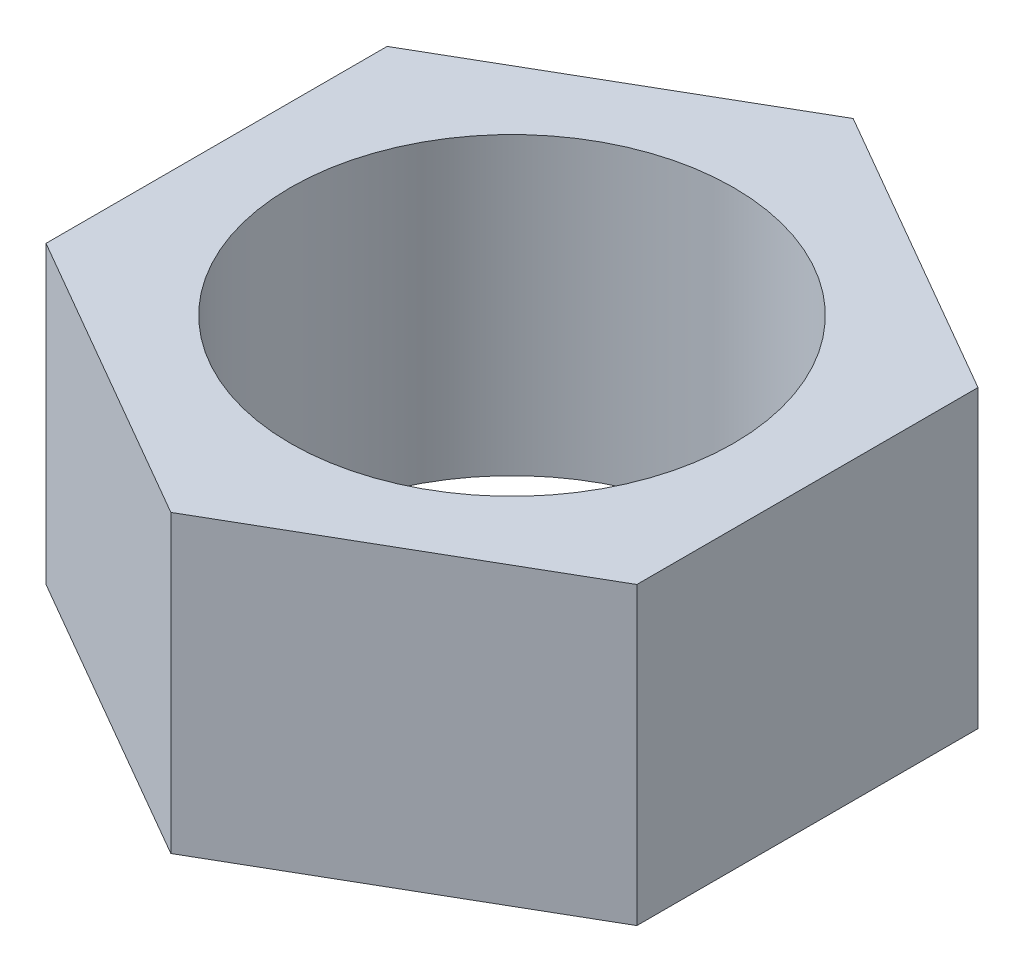
ISO-10303-21;
HEADER;
FILE_DESCRIPTION(('STEP AP214'),'2;1');
FILE_NAME('part.step','',(''),(''),'','','');
FILE_SCHEMA(('AUTOMOTIVE_DESIGN { 1 0 10303 214 1 1 1 1 }'));
ENDSEC;
DATA;
#1=APPLICATION_CONTEXT('core data for automotive mechanical design processes');
#2=APPLICATION_PROTOCOL_DEFINITION('international standard','automotive_design',2000,#1);
#3=PRODUCT_CONTEXT('',#1,'mechanical');
#4=PRODUCT('Part','Part','',(#3));
#5=PRODUCT_RELATED_PRODUCT_CATEGORY('part','',(#4));
#6=PRODUCT_DEFINITION_FORMATION('','',#4);
#7=PRODUCT_DEFINITION_CONTEXT('part definition',#1,'design');
#8=PRODUCT_DEFINITION('design','',#6,#7);
#9=PRODUCT_DEFINITION_SHAPE('','',#8);
#10=(LENGTH_UNIT() NAMED_UNIT(*) SI_UNIT(.MILLI.,.METRE.));
#11=(NAMED_UNIT(*) PLANE_ANGLE_UNIT() SI_UNIT($,.RADIAN.));
#12=(NAMED_UNIT(*) SI_UNIT($,.STERADIAN.) SOLID_ANGLE_UNIT());
#13=UNCERTAINTY_MEASURE_WITH_UNIT(LENGTH_MEASURE(1.E-05),#10,'distance_accuracy_value','');
#14=(GEOMETRIC_REPRESENTATION_CONTEXT(3) GLOBAL_UNCERTAINTY_ASSIGNED_CONTEXT((#13)) GLOBAL_UNIT_ASSIGNED_CONTEXT((#10,
#11,#12)) REPRESENTATION_CONTEXT('',''));
#15=CARTESIAN_POINT('',(0.,0.,0.));
#16=DIRECTION('',(0.,0.,1.));
#17=DIRECTION('',(1.,0.,0.));
#18=AXIS2_PLACEMENT_3D('',#15,#16,#17);
#19=CARTESIAN_POINT('',(0.,4.,0.));
#20=DIRECTION('',(0.,1.,0.));
#21=DIRECTION('',(0.,0.,1.));
#22=AXIS2_PLACEMENT_3D('',#19,#20,#21);
#23=PLANE('',#22);
#24=DIRECTION('',(0.866025403784438,0.,0.5));
#25=VECTOR('',#24,1.);
#26=CARTESIAN_POINT('',(-8.,4.,4.61880215351701));
#27=LINE('',#26,#25);
#28=CARTESIAN_POINT('',(-8.,4.,4.61880215351701));
#29=VERTEX_POINT('',#28);
#30=CARTESIAN_POINT('',(0.,4.,9.23760430703401));
#31=VERTEX_POINT('',#30);
#32=EDGE_CURVE('E132',#29,#31,#27,.T.);
#33=ORIENTED_EDGE('',*,*,#32,.T.);
#34=DIRECTION('',(0.866025403784439,0.,-0.5));
#35=VECTOR('',#34,1.);
#36=CARTESIAN_POINT('',(0.,4.,9.23760430703401));
#37=LINE('',#36,#35);
#38=CARTESIAN_POINT('',(8.,4.,4.61880215351701));
#39=VERTEX_POINT('',#38);
#40=EDGE_CURVE('E91',#31,#39,#37,.T.);
#41=ORIENTED_EDGE('',*,*,#40,.T.);
#42=DIRECTION('',(0.,0.,-1.));
#43=VECTOR('',#42,1.);
#44=CARTESIAN_POINT('',(8.,4.,4.61880215351701));
#45=LINE('',#44,#43);
#46=CARTESIAN_POINT('',(7.9999999999999,4.,-4.61880215351684));
#47=VERTEX_POINT('',#46);
#48=EDGE_CURVE('E106',#39,#47,#45,.T.);
#49=ORIENTED_EDGE('',*,*,#48,.T.);
#50=DIRECTION('',(-0.866025403784428,0.,-0.500000000000018));
#51=VECTOR('',#50,1.);
#52=CARTESIAN_POINT('',(7.9999999999999,4.,-4.61880215351684));
#53=LINE('',#52,#51);
#54=CARTESIAN_POINT('',(0.,4.,-9.23760430703401));
#55=VERTEX_POINT('',#54);
#56=EDGE_CURVE('E99',#47,#55,#53,.T.);
#57=ORIENTED_EDGE('',*,*,#56,.T.);
#58=DIRECTION('',(-0.866025403784439,0.,0.5));
#59=VECTOR('',#58,1.);
#60=CARTESIAN_POINT('',(0.,4.,-9.23760430703401));
#61=LINE('',#60,#59);
#62=CARTESIAN_POINT('',(-8.,4.,-4.61880215351701));
#63=VERTEX_POINT('',#62);
#64=EDGE_CURVE('E102',#55,#63,#61,.T.);
#65=ORIENTED_EDGE('',*,*,#64,.T.);
#66=DIRECTION('',(0.,0.,1.));
#67=VECTOR('',#66,1.);
#68=CARTESIAN_POINT('',(-8.,4.,-4.61880215351701));
#69=LINE('',#68,#67);
#70=EDGE_CURVE('E57',#63,#29,#69,.T.);
#71=ORIENTED_EDGE('',*,*,#70,.T.);
#72=EDGE_LOOP('',(#33,#41,#49,#57,#65,#71));
#73=FACE_BOUND('',#72,.T.);
#74=CARTESIAN_POINT('',(0.,4.,0.));
#75=DIRECTION('',(0.,1.,0.));
#76=DIRECTION('',(0.,0.,1.));
#77=AXIS2_PLACEMENT_3D('',#74,#75,#76);
#78=CIRCLE('',#77,6.00000000000001);
#79=CARTESIAN_POINT('',(0.,4.,6.00000000000001));
#80=VERTEX_POINT('',#79);
#81=EDGE_CURVE('E126',#80,#80,#78,.T.);
#82=ORIENTED_EDGE('',*,*,#81,.F.);
#83=EDGE_LOOP('',(#82));
#84=FACE_BOUND('',#83,.T.);
#85=ADVANCED_FACE('F39',(#73,#84),#23,.T.);
#86=CARTESIAN_POINT('',(0.,-4.,0.));
#87=DIRECTION('',(0.,1.,0.));
#88=DIRECTION('',(0.,0.,1.));
#89=AXIS2_PLACEMENT_3D('',#86,#87,#88);
#90=PLANE('',#89);
#91=DIRECTION('',(0.866025403784438,0.,0.5));
#92=VECTOR('',#91,1.);
#93=CARTESIAN_POINT('',(-8.,-4.,4.61880215351701));
#94=LINE('',#93,#92);
#95=CARTESIAN_POINT('',(-8.,-4.,4.61880215351701));
#96=VERTEX_POINT('',#95);
#97=CARTESIAN_POINT('',(0.,-4.,9.23760430703401));
#98=VERTEX_POINT('',#97);
#99=EDGE_CURVE('E122',#96,#98,#94,.T.);
#100=ORIENTED_EDGE('',*,*,#99,.F.);
#101=DIRECTION('',(0.,0.,1.));
#102=VECTOR('',#101,1.);
#103=CARTESIAN_POINT('',(-8.,-4.,-4.61880215351701));
#104=LINE('',#103,#102);
#105=CARTESIAN_POINT('',(-8.,-4.,-4.61880215351701));
#106=VERTEX_POINT('',#105);
#107=EDGE_CURVE('E84',#106,#96,#104,.T.);
#108=ORIENTED_EDGE('',*,*,#107,.F.);
#109=DIRECTION('',(-0.866025403784439,0.,0.5));
#110=VECTOR('',#109,1.);
#111=CARTESIAN_POINT('',(0.,-4.,-9.23760430703401));
#112=LINE('',#111,#110);
#113=CARTESIAN_POINT('',(0.,-4.,-9.23760430703401));
#114=VERTEX_POINT('',#113);
#115=EDGE_CURVE('E78',#114,#106,#112,.T.);
#116=ORIENTED_EDGE('',*,*,#115,.F.);
#117=DIRECTION('',(-0.866025403784428,0.,-0.500000000000018));
#118=VECTOR('',#117,1.);
#119=CARTESIAN_POINT('',(7.9999999999999,-4.,-4.61880215351684));
#120=LINE('',#119,#118);
#121=CARTESIAN_POINT('',(7.9999999999999,-4.,-4.61880215351684));
#122=VERTEX_POINT('',#121);
#123=EDGE_CURVE('E111',#122,#114,#120,.T.);
#124=ORIENTED_EDGE('',*,*,#123,.F.);
#125=DIRECTION('',(0.,0.,-1.));
#126=VECTOR('',#125,1.);
#127=CARTESIAN_POINT('',(8.,-4.,4.61880215351701));
#128=LINE('',#127,#126);
#129=CARTESIAN_POINT('',(8.,-4.,4.61880215351701));
#130=VERTEX_POINT('',#129);
#131=EDGE_CURVE('E128',#130,#122,#128,.T.);
#132=ORIENTED_EDGE('',*,*,#131,.F.);
#133=DIRECTION('',(0.866025403784439,0.,-0.5));
#134=VECTOR('',#133,1.);
#135=CARTESIAN_POINT('',(0.,-4.,9.23760430703401));
#136=LINE('',#135,#134);
#137=EDGE_CURVE('E130',#98,#130,#136,.T.);
#138=ORIENTED_EDGE('',*,*,#137,.F.);
#139=EDGE_LOOP('',(#100,#108,#116,#124,#132,#138));
#140=FACE_BOUND('',#139,.T.);
#141=CARTESIAN_POINT('',(0.,-4.,0.));
#142=DIRECTION('',(0.,1.,0.));
#143=DIRECTION('',(0.,0.,1.));
#144=AXIS2_PLACEMENT_3D('',#141,#142,#143);
#145=CIRCLE('',#144,6.00000000000001);
#146=CARTESIAN_POINT('',(0.,-4.,6.00000000000001));
#147=VERTEX_POINT('',#146);
#148=EDGE_CURVE('E230',#147,#147,#145,.T.);
#149=ORIENTED_EDGE('',*,*,#148,.T.);
#150=EDGE_LOOP('',(#149));
#151=FACE_BOUND('',#150,.T.);
#152=ADVANCED_FACE('F145',(#140,#151),#90,.F.);
#153=CARTESIAN_POINT('',(-8.,4.,4.61880215351701));
#154=DIRECTION('',(0.5,0.,-0.866025403784439));
#155=DIRECTION('',(-0.866025403784439,0.,-0.5));
#156=AXIS2_PLACEMENT_3D('',#153,#154,#155);
#157=PLANE('',#156);
#158=ORIENTED_EDGE('',*,*,#99,.T.);
#159=DIRECTION('',(0.,-1.,0.));
#160=VECTOR('',#159,1.);
#161=CARTESIAN_POINT('',(0.,4.,9.23760430703401));
#162=LINE('',#161,#160);
#163=EDGE_CURVE('E11',#31,#98,#162,.T.);
#164=ORIENTED_EDGE('',*,*,#163,.F.);
#165=ORIENTED_EDGE('',*,*,#32,.F.);
#166=DIRECTION('',(0.,-1.,0.));
#167=VECTOR('',#166,1.);
#168=CARTESIAN_POINT('',(-8.,4.,4.61880215351701));
#169=LINE('',#168,#167);
#170=EDGE_CURVE('E117',#29,#96,#169,.T.);
#171=ORIENTED_EDGE('',*,*,#170,.T.);
#172=EDGE_LOOP('',(#158,#164,#165,#171));
#173=FACE_BOUND('',#172,.T.);
#174=ADVANCED_FACE('F41',(#173),#157,.F.);
#175=CARTESIAN_POINT('',(0.,4.,9.23760430703401));
#176=DIRECTION('',(-0.5,0.,-0.866025403784439));
#177=DIRECTION('',(-0.866025403784439,0.,0.5));
#178=AXIS2_PLACEMENT_3D('',#175,#176,#177);
#179=PLANE('',#178);
#180=ORIENTED_EDGE('',*,*,#137,.T.);
#181=DIRECTION('',(0.,-1.,0.));
#182=VECTOR('',#181,1.);
#183=CARTESIAN_POINT('',(8.,4.,4.61880215351701));
#184=LINE('',#183,#182);
#185=EDGE_CURVE('E48',#39,#130,#184,.T.);
#186=ORIENTED_EDGE('',*,*,#185,.F.);
#187=ORIENTED_EDGE('',*,*,#40,.F.);
#188=ORIENTED_EDGE('',*,*,#163,.T.);
#189=EDGE_LOOP('',(#180,#186,#187,#188));
#190=FACE_BOUND('',#189,.T.);
#191=ADVANCED_FACE('F166',(#190),#179,.F.);
#192=CARTESIAN_POINT('',(8.,4.,4.61880215351701));
#193=DIRECTION('',(-1.,0.,0.));
#194=DIRECTION('',(0.,0.,1.));
#195=AXIS2_PLACEMENT_3D('',#192,#193,#194);
#196=PLANE('',#195);
#197=ORIENTED_EDGE('',*,*,#131,.T.);
#198=DIRECTION('',(0.,-1.,0.));
#199=VECTOR('',#198,1.);
#200=CARTESIAN_POINT('',(7.9999999999999,4.,-4.61880215351684));
#201=LINE('',#200,#199);
#202=EDGE_CURVE('E113',#47,#122,#201,.T.);
#203=ORIENTED_EDGE('',*,*,#202,.F.);
#204=ORIENTED_EDGE('',*,*,#48,.F.);
#205=ORIENTED_EDGE('',*,*,#185,.T.);
#206=EDGE_LOOP('',(#197,#203,#204,#205));
#207=FACE_BOUND('',#206,.T.);
#208=ADVANCED_FACE('F143',(#207),#196,.F.);
#209=CARTESIAN_POINT('',(7.9999999999999,4.,-4.61880215351684));
#210=DIRECTION('',(-0.500000000000018,0.,0.866025403784428));
#211=DIRECTION('',(0.866025403784428,0.,0.500000000000018));
#212=AXIS2_PLACEMENT_3D('',#209,#210,#211);
#213=PLANE('',#212);
#214=ORIENTED_EDGE('',*,*,#123,.T.);
#215=DIRECTION('',(0.,-1.,0.));
#216=VECTOR('',#215,1.);
#217=CARTESIAN_POINT('',(0.,4.,-9.23760430703401));
#218=LINE('',#217,#216);
#219=EDGE_CURVE('E112',#55,#114,#218,.T.);
#220=ORIENTED_EDGE('',*,*,#219,.F.);
#221=ORIENTED_EDGE('',*,*,#56,.F.);
#222=ORIENTED_EDGE('',*,*,#202,.T.);
#223=EDGE_LOOP('',(#214,#220,#221,#222));
#224=FACE_BOUND('',#223,.T.);
#225=ADVANCED_FACE('F115',(#224),#213,.F.);
#226=CARTESIAN_POINT('',(0.,4.,-9.23760430703401));
#227=DIRECTION('',(0.5,0.,0.866025403784439));
#228=DIRECTION('',(0.866025403784439,0.,-0.5));
#229=AXIS2_PLACEMENT_3D('',#226,#227,#228);
#230=PLANE('',#229);
#231=ORIENTED_EDGE('',*,*,#115,.T.);
#232=DIRECTION('',(0.,-1.,0.));
#233=VECTOR('',#232,1.);
#234=CARTESIAN_POINT('',(-8.,4.,-4.61880215351701));
#235=LINE('',#234,#233);
#236=EDGE_CURVE('E119',#63,#106,#235,.T.);
#237=ORIENTED_EDGE('',*,*,#236,.F.);
#238=ORIENTED_EDGE('',*,*,#64,.F.);
#239=ORIENTED_EDGE('',*,*,#219,.T.);
#240=EDGE_LOOP('',(#231,#237,#238,#239));
#241=FACE_BOUND('',#240,.T.);
#242=ADVANCED_FACE('F120',(#241),#230,.F.);
#243=CARTESIAN_POINT('',(-8.,4.,-4.61880215351701));
#244=DIRECTION('',(1.,0.,0.));
#245=DIRECTION('',(0.,0.,-1.));
#246=AXIS2_PLACEMENT_3D('',#243,#244,#245);
#247=PLANE('',#246);
#248=ORIENTED_EDGE('',*,*,#107,.T.);
#249=ORIENTED_EDGE('',*,*,#170,.F.);
#250=ORIENTED_EDGE('',*,*,#70,.F.);
#251=ORIENTED_EDGE('',*,*,#236,.T.);
#252=EDGE_LOOP('',(#248,#249,#250,#251));
#253=FACE_BOUND('',#252,.T.);
#254=ADVANCED_FACE('F149',(#253),#247,.F.);
#255=CARTESIAN_POINT('',(0.,4.,0.));
#256=DIRECTION('',(0.,-1.,0.));
#257=DIRECTION('',(0.,0.,-1.));
#258=AXIS2_PLACEMENT_3D('',#255,#256,#257);
#259=CYLINDRICAL_SURFACE('',#258,6.00000000000001);
#260=ORIENTED_EDGE('',*,*,#81,.T.);
#261=EDGE_LOOP('',(#260));
#262=FACE_BOUND('',#261,.T.);
#263=ORIENTED_EDGE('',*,*,#148,.F.);
#264=EDGE_LOOP('',(#263));
#265=FACE_BOUND('',#264,.T.);
#266=ADVANCED_FACE('F151',(#262,#265),#259,.F.);
#267=CLOSED_SHELL('',(#85,#152,#174,#191,#208,#225,#242,#254,#266));
#268=MANIFOLD_SOLID_BREP('B2',#267);
#269=ADVANCED_BREP_SHAPE_REPRESENTATION('',(#18,#268),#14);
#270=SHAPE_DEFINITION_REPRESENTATION(#9,#269);
ENDSEC;
END-ISO-10303-21;
